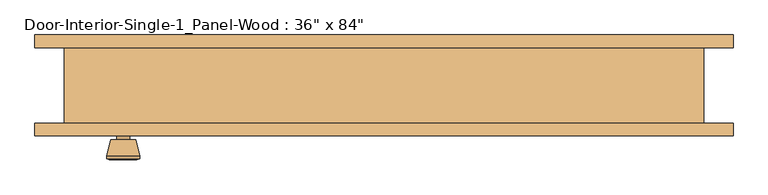
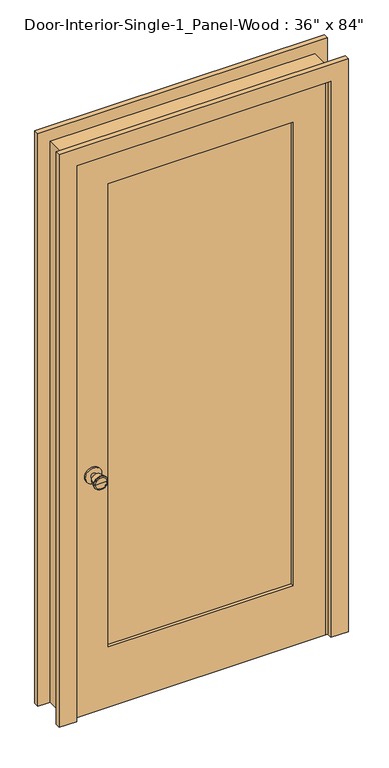
"""IFC4 building model written with IfcOpenShell, lengths in millimetres: door geometry."""

from ifc_helpers import new_model, si_unit, point, frame, frame_2d, origin, place, context, project, spatial, polyline, circle_curve, trimmed, segment, composite_curve, outline, extrude, faceted_brep, source, transform, mapped, element, save
from ifc_brep_helpers import plane_surface, cylinder_surface, revolved_surface, advanced_brep


def door_a3feeac7(model_context):
    return source(origin(), model_context, "Body", "SolidModel", [
        advanced_brep(
        [(-393.7, -13.05, 914.4), (-403.7, -13.05, 914.4), (-383.7, -13.05, 914.4), (-373.2241324, 35.95, 914.4), (-414.1758676, 35.95, 914.4), (-393.7, 35.95, 914.4), (-368.7, 34.1221319, 914.4), (-418.7, 34.1221319, 914.4), (-368.7, 30.6584537, 914.4), (-418.7, 30.6584537, 914.4), (-375.063764, 5.95, 914.4), (-412.336236, 5.95, 914.4), (-383.7, 5.95, 914.4), (-403.7, 5.95, 914.4)],
        [
            (0, 1),
            (1, 2, circle_curve(frame((-393.7, -13.05, 914.4), z_axis=(0.0, -1.0, 0.0), x_axis=(-1.0, 0.0, 0.0)), 10.0)),
            (2, 0),
            (2, 1, circle_curve(frame((-393.7, -13.05, 914.4), z_axis=(0.0, -1.0, 0.0), x_axis=(-1.0, 0.0, 0.0)), 10.0)),
            (3, 4, circle_curve(frame((-393.7, 35.95, 914.4), z_axis=(0.0, 1.0, 0.0), x_axis=(-1.0, 0.0, 0.0)), 20.4758676)),
            (4, 5),
            (5, 3),
            (4, 3, circle_curve(frame((-393.7, 35.95, 914.4), z_axis=(0.0, 1.0, 0.0), x_axis=(-1.0, 0.0, 0.0)), 20.4758676)),
            (6, 7, circle_curve(frame((-393.7, 34.1221319, 914.4), z_axis=(0.0, 1.0, 0.0), x_axis=(-1.0, 0.0, 0.0)), 25.0)),
            (7, 4),
            (3, 6),
            (7, 6, circle_curve(frame((-393.7, 34.1221319, 914.4), z_axis=(0.0, 1.0, 0.0), x_axis=(-1.0, 0.0, 0.0)), 25.0)),
            (8, 9, circle_curve(frame((-393.7, 30.6584537, 914.4), z_axis=(0.0, 1.0, 0.0), x_axis=(-1.0, 0.0, 0.0)), 25.0)),
            (9, 7),
            (6, 8),
            (9, 8, circle_curve(frame((-393.7, 30.6584537, 914.4), z_axis=(0.0, 1.0, 0.0), x_axis=(-1.0, 0.0, 0.0)), 25.0)),
            (10, 11, circle_curve(frame((-393.7, 5.95, 914.4), z_axis=(0.0, 1.0, 0.0), x_axis=(-1.0, 0.0, 0.0)), 18.636236)),
            (11, 9),
            (8, 10),
            (11, 10, circle_curve(frame((-393.7, 5.95, 914.4), z_axis=(0.0, 1.0, 0.0), x_axis=(-1.0, 0.0, 0.0)), 18.636236)),
            (12, 13, circle_curve(frame((-393.7, 5.95, 914.4), z_axis=(0.0, 1.0, 0.0), x_axis=(-1.0, 0.0, 0.0)), 10.0)),
            (13, 11),
            (10, 12),
            (13, 12, circle_curve(frame((-393.7, 5.95, 914.4), z_axis=(0.0, 1.0, 0.0), x_axis=(-1.0, 0.0, 0.0)), 10.0)),
            (1, 13),
            (12, 2),
        ],
        [
            plane_surface(frame((-393.7, -13.05, 914.4), z_axis=(0.0, -1.0, 0.0), x_axis=(-1.0, 0.0, 0.0))),
            plane_surface(frame((-393.7, 35.95, 914.4), z_axis=(0.0, 1.0, 0.0), x_axis=(-1.0, 0.0, 0.0))),
            revolved_surface(polyline([(-414.1758676, 35.95, 914.4), (-418.7, 34.1221319, 914.4)]), (-393.7, -13.05, 914.4), (0.0, -1.0, 0.0)),
            cylinder_surface(frame((-393.7, -13.05, 914.4), z_axis=(0.0, -1.0, 0.0), x_axis=(-1.0, 0.0, 0.0)), 25.0),
            revolved_surface(polyline([(-418.7, 30.6584537, 914.4), (-412.336236, 5.95, 914.4)]), (-393.7, -13.05, 914.4), (0.0, -1.0, 0.0)),
            plane_surface(frame((-393.7, 5.95, 914.4), z_axis=(0.0, -1.0, 0.0), x_axis=(-1.0, 0.0, 0.0))),
            cylinder_surface(frame((-393.7, -13.05, 914.4), z_axis=(0.0, -1.0, 0.0), x_axis=(-1.0, 0.0, 0.0)), 10.0),
        ],
        [
            (0, [[1, 2, 3]]),
            (0, [[-3, 4, -1]]),
            (1, [[5, 6, 7]]),
            (1, [[8, -7, -6]]),
            (2, [[9, 10, -5, 11]]),
            (2, [[12, -11, -8, -10]]),
            (3, [[13, 14, -9, 15]]),
            (3, [[16, -15, -12, -14]]),
            (4, [[17, 18, -13, 19]]),
            (4, [[20, -19, -16, -18]]),
            (5, [[21, 22, -17, 23]]),
            (5, [[24, -23, -20, -22]]),
            (6, [[-2, 25, -21, 26]]),
            (6, [[-4, -26, -24, -25]]),
        ],
    ),
        extrude(outline(composite_curve([segment(trimmed(circle_curve(frame_2d((914.4, -393.7)), 30.0), [point((914.4, -423.7))], [point((914.4, -363.7))], False, "CARTESIAN"), True, "CONTINUOUS"), segment(trimmed(circle_curve(frame_2d((914.4, -393.7)), 30.0), [point((914.4, -363.7))], [point((914.4, -423.7))], False, "CARTESIAN"), True, "CONTINUOUS")], self_intersect=False)), frame((0.0, -19.05, 0.0), z_axis=(0.0, 1.0, 0.0), x_axis=(0.0, 0.0, 1.0)), (0.0, 0.0, 1.0), 6.0),
        advanced_brep(
        [(-393.7, -59.975, 914.4), (-383.7, -59.975, 914.4), (-403.7, -59.975, 914.4), (-373.2241324, -108.975, 914.4), (-393.7, -108.975, 914.4), (-414.1758676, -108.975, 914.4), (-368.7, -107.1471319, 914.4), (-418.7, -107.1471319, 914.4), (-368.7, -103.6834537, 914.4), (-418.7, -103.6834537, 914.4), (-375.063764, -78.975, 914.4), (-412.336236, -78.975, 914.4), (-383.7, -78.975, 914.4), (-403.7, -78.975, 914.4)],
        [
            (0, 1),
            (1, 2, circle_curve(frame((-393.7, -59.975, 914.4), z_axis=(0.0, 1.0, 0.0), x_axis=(-1.0, 0.0, 0.0)), 10.0)),
            (2, 0),
            (2, 1, circle_curve(frame((-393.7, -59.975, 914.4), z_axis=(0.0, 1.0, 0.0), x_axis=(-1.0, 0.0, 0.0)), 10.0)),
            (3, 4),
            (4, 5),
            (5, 3, circle_curve(frame((-393.7, -108.975, 914.4), z_axis=(0.0, -1.0, 0.0), x_axis=(-1.0, 0.0, 0.0)), 20.4758676)),
            (3, 5, circle_curve(frame((-393.7, -108.975, 914.4), z_axis=(0.0, -1.0, 0.0), x_axis=(-1.0, 0.0, 0.0)), 20.4758676)),
            (6, 3),
            (5, 7),
            (7, 6, circle_curve(frame((-393.7, -107.1471319, 914.4), z_axis=(0.0, -1.0, 0.0), x_axis=(-1.0, 0.0, 0.0)), 25.0)),
            (6, 7, circle_curve(frame((-393.7, -107.1471319, 914.4), z_axis=(0.0, -1.0, 0.0), x_axis=(-1.0, 0.0, 0.0)), 25.0)),
            (8, 6),
            (7, 9),
            (9, 8, circle_curve(frame((-393.7, -103.6834537, 914.4), z_axis=(0.0, -1.0, 0.0), x_axis=(-1.0, 0.0, 0.0)), 25.0)),
            (8, 9, circle_curve(frame((-393.7, -103.6834537, 914.4), z_axis=(0.0, -1.0, 0.0), x_axis=(-1.0, 0.0, 0.0)), 25.0)),
            (10, 8),
            (9, 11),
            (11, 10, circle_curve(frame((-393.7, -78.975, 914.4), z_axis=(0.0, -1.0, 0.0), x_axis=(-1.0, 0.0, 0.0)), 18.636236)),
            (10, 11, circle_curve(frame((-393.7, -78.975, 914.4), z_axis=(0.0, -1.0, 0.0), x_axis=(-1.0, 0.0, 0.0)), 18.636236)),
            (12, 10),
            (11, 13),
            (13, 12, circle_curve(frame((-393.7, -78.975, 914.4), z_axis=(0.0, -1.0, 0.0), x_axis=(-1.0, 0.0, 0.0)), 10.0)),
            (12, 13, circle_curve(frame((-393.7, -78.975, 914.4), z_axis=(0.0, -1.0, 0.0), x_axis=(-1.0, 0.0, 0.0)), 10.0)),
            (1, 12),
            (13, 2),
        ],
        [
            plane_surface(frame((-393.7, -59.975, 914.4), z_axis=(0.0, 1.0, 0.0), x_axis=(-1.0, 0.0, 0.0))),
            plane_surface(frame((-393.7, -108.975, 914.4), z_axis=(0.0, -1.0, 0.0), x_axis=(-1.0, 0.0, 0.0))),
            revolved_surface(polyline([(-414.1758676, -108.975, 914.4), (-418.7, -107.1471319, 914.4)]), (-393.7, -59.975, 914.4), (0.0, 1.0, 0.0)),
            cylinder_surface(frame((-393.7, -59.975, 914.4), z_axis=(0.0, 1.0, 0.0), x_axis=(-1.0, 0.0, 0.0)), 25.0),
            revolved_surface(polyline([(-418.7, -103.6834537, 914.4), (-412.336236, -78.975, 914.4)]), (-393.7, -59.975, 914.4), (0.0, 1.0, 0.0)),
            plane_surface(frame((-393.7, -78.975, 914.4), z_axis=(0.0, 1.0, 0.0), x_axis=(-1.0, 0.0, 0.0))),
            cylinder_surface(frame((-393.7, -59.975, 914.4), z_axis=(0.0, 1.0, 0.0), x_axis=(-1.0, 0.0, 0.0)), 10.0),
        ],
        [
            (0, [[1, 2, 3]]),
            (0, [[-3, 4, -1]]),
            (1, [[5, 6, 7]]),
            (1, [[-6, -5, 8]]),
            (2, [[9, -7, 10, 11]]),
            (2, [[-10, -8, -9, 12]]),
            (3, [[13, -11, 14, 15]]),
            (3, [[-14, -12, -13, 16]]),
            (4, [[17, -15, 18, 19]]),
            (4, [[-18, -16, -17, 20]]),
            (5, [[21, -19, 22, 23]]),
            (5, [[-22, -20, -21, 24]]),
            (6, [[25, -23, 26, -2]]),
            (6, [[-26, -24, -25, -4]]),
        ],
    ),
        extrude(outline(composite_curve([segment(trimmed(circle_curve(frame_2d((914.4, -393.7)), 30.0), [point((914.4, -423.7))], [point((914.4, -363.7))], False, "CARTESIAN"), True, "CONTINUOUS"), segment(trimmed(circle_curve(frame_2d((914.4, -393.7)), 30.0), [point((914.4, -363.7))], [point((914.4, -423.7))], False, "CARTESIAN"), True, "CONTINUOUS")], self_intersect=False)), frame((0.0, -59.975, 0.0), z_axis=(0.0, 1.0, 0.0), x_axis=(0.0, 0.0, 1.0)), (0.0, 0.0, 1.0), 6.0),
        faceted_brep([(482.6, -53.975, 0.0), (457.2, -53.975, 0.0), (457.2, -19.05, 0.0), (444.5, -19.05, 0.0), (444.5, 15.875, 0.0), (457.2, 15.875, 0.0), (457.2, 60.325, 0.0), (482.6, 60.325, 0.0), (482.6, 60.325, 2159.0), (482.6, -53.975, 2159.0), (457.2, 60.325, 2133.6), (-457.2, 60.325, 2133.6), (-457.2, 60.325, 0.0), (-482.6, 60.325, 0.0), (-482.6, 60.325, 2159.0), (457.2, 15.875, 2133.6), (444.5, 15.875, 2120.9), (-444.5, 15.875, 2120.9), (-444.5, 15.875, 0.0), (-457.2, 15.875, 0.0), (-457.2, 15.875, 2133.6), (444.5, -19.05, 2120.9), (457.2, -19.05, 2133.6), (-457.2, -19.05, 2133.6), (-457.2, -19.05, 0.0), (-444.5, -19.05, 0.0), (-444.5, -19.05, 2120.9), (457.2, -53.975, 2133.6), (-482.6, -53.975, 2159.0), (-482.6, -53.975, 0.0), (-457.2, -53.975, 0.0), (-457.2, -53.975, 2133.6)], [[[0, 1, 2, 3, 4, 5, 6, 7]], [[7, 8, 9, 0]], [[6, 10, 11, 12, 13, 14, 8, 7]], [[5, 15, 10, 6]], [[4, 16, 17, 18, 19, 20, 15, 5]], [[3, 21, 16, 4]], [[2, 22, 23, 24, 25, 26, 21, 3]], [[1, 27, 22, 2]], [[0, 9, 28, 29, 30, 31, 27, 1]], [[8, 14, 28, 9]], [[15, 20, 11, 10]], [[21, 26, 17, 16]], [[27, 31, 23, 22]], [[29, 13, 12, 19, 18, 25, 24, 30]], [[14, 13, 29, 28]], [[20, 19, 12, 11]], [[26, 25, 18, 17]], [[31, 30, 24, 23]]]),
        extrude(outline(polyline([(2133.6, -457.2), (0.0, -457.2), (0.0, 457.2), (2133.6, 457.2), (2133.6, -457.2)]), holes=[polyline([(2014.5375, -336.55), (2014.5375, 336.55), (231.775, 336.55), (231.775, -336.55), (2014.5375, -336.55)])]), frame((0.0, -53.975, 0.0), z_axis=(0.0, 1.0, 0.0), x_axis=(0.0, 0.0, 1.0)), (0.0, 0.0, 1.0), 34.925),
        extrude(outline(polyline([(336.55, -30.6916667), (336.55, -42.3333333), (-336.55, -42.3333333), (-336.55, -30.6916667), (336.55, -30.6916667)])), frame((0.0, 0.0, 231.775), z_axis=(0.0, 0.0, 1.0), x_axis=(1.0, 0.0, 0.0)), (0.0, 0.0, 1.0), 1782.7625),
        extrude(outline(polyline([(0.0, 527.05), (2203.45, 527.05), (2203.45, -527.05), (0.0, -527.05), (0.0, -463.55), (2139.95, -463.55), (2139.95, 463.55), (0.0, 463.55), (0.0, 527.05)])), frame((0.0, -73.025, 0.0), z_axis=(0.0, 1.0, 0.0), x_axis=(0.0, 0.0, 1.0)), (0.0, 0.0, 1.0), 19.05),
        extrude(outline(polyline([(0.0, 527.05), (2203.45, 527.05), (2203.45, -527.05), (0.0, -527.05), (0.0, -463.55), (2139.95, -463.55), (2139.95, 463.55), (0.0, 463.55), (0.0, 527.05)])), frame((0.0, 60.325, 0.0), z_axis=(0.0, 1.0, 0.0), x_axis=(0.0, 0.0, 1.0)), (0.0, 0.0, 1.0), 19.05),
    ])


if __name__ == "__main__":
    model = new_model("IFC4")
    model_context = context("Model", 3, world=origin())
    ifc_project = project(units=[si_unit("LENGTHUNIT", "METRE", prefix="MILLI")], contexts=[model_context])
    site = spatial("IfcSite", under=ifc_project)
    building = spatial("IfcBuilding", under=site)
    placement = place(None, origin())
    door_shape = door_a3feeac7(model_context)
    element("IfcDoor", 1, ObjectType="Door-Interior-Single-1_Panel-Wood : 36\" x 84\"", at=placement, inside=building, context=model_context, shape_type="MappedRepresentation", body=[
        mapped(door_shape, transform((0.0, 0.0, 0.0), x_axis=(1.0, 0.0, 0.0), y_axis=(0.0, 1.0, 0.0), z_axis=(0.0, 0.0, 1.0))),
    ])
    save(model, "model.ifc")

# Revit data of these elements
# Type "Door-Interior-Single-1_Panel-Wood : 36\" x 84\""
#   Type Mark = "10"
#   Assembly Code = "C1020300"
#   Analytic Construction = "Wooden"
#   Top Rail = 0' - 4 11/16"
#   Thickness = 0' - 1 3/8"
#   Thermal Resistance (R) = 2.5876 (h·ft²·°F)/BTU
#   Swing Angle [instance default] = 90.00°
#   Stiles = 0' - 4 3/4"
#   Rough Width = 3' - 2"
#   Rough Height = 7' - 1"
#   Height = 7' - 0"
#   Width = 3' - 0"
#   Heat Transfer Coefficient (U) = 0.3865 BTU/(h·ft²·°F)
#   Bottom Rail = 0' - 9 1/8"
#   Trim Material = Cherry
#   Panel Material = Cherry
#   Frame Material = Cherry
#   Door Handle Material = Aluminum
#   Visual Light Transmittance = 0
#   Solar Heat Gain Coefficient = 0
#   Wall Closure = (empty or 0)
#   Function = (empty or 0)
# Element 1 (IfcDoor, "Door-Interior-Single-1_Panel-Wood : 36\" x 84\"")
#   Materials on its faces: "Cherry", "Aluminum"
# Materials
#   "Cherry": class "Wood", colour RGB 226 177 128, transparency 0, Description = "Prunus Serotina", Cost = 0
#   "Aluminum": class "Metal", colour RGB 247 247 247, transparency 0, Description = "Aluminum 6061", Cost = 0
